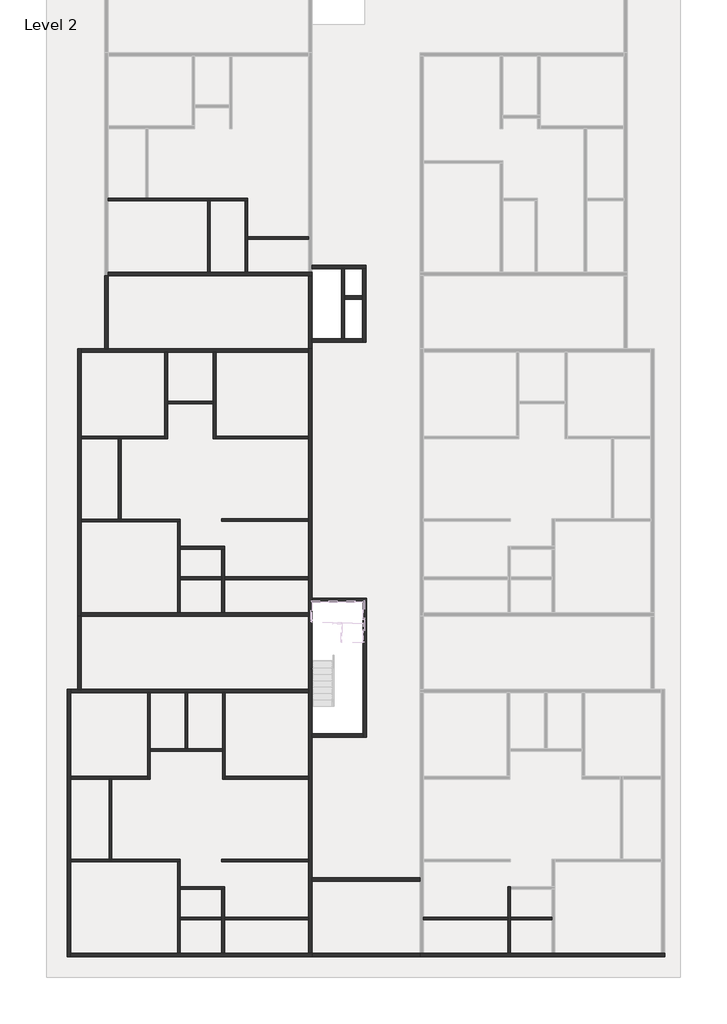
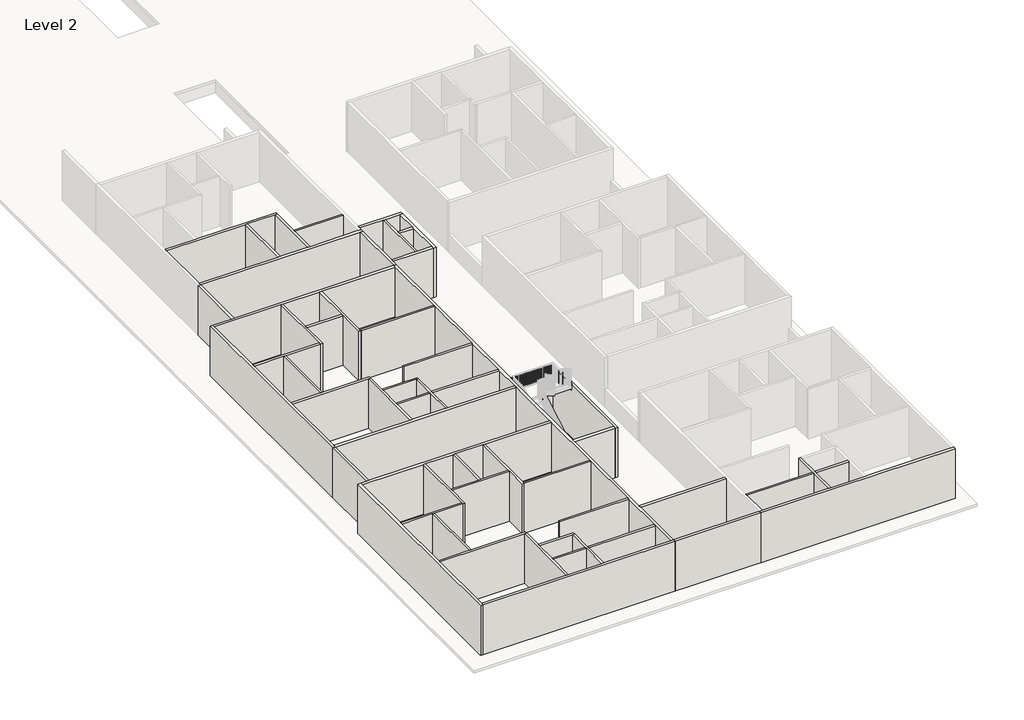
# One storey, part 1 of 8: 55 walls.
"""IFC4 building model written with IfcOpenShell, lengths in millimetres."""

from ifc_helpers import new_model, si_unit, frame, origin, place, context, project, spatial, polyline, outline, extrude, faceted_brep, element, save

model = new_model("IFC4")

# Units and contexts
model_context = context("Model", 3, world=origin())
ifc_project = project(units=[si_unit("LENGTHUNIT", "METRE", prefix="MILLI")], contexts=[model_context])

# Site, building, storey
site = spatial("IfcSite", under=ifc_project)
building = spatial("IfcBuilding", under=site)
storey = spatial("IfcBuildingStorey", under=building, Name="Level 2", Elevation=28282.6172466)

# Walls
placement = place(None, origin())
element("IfcWall", 1, ObjectType="4.5\"", at=placement, inside=storey, context=model_context, shape_type="Brep", body=[
    faceted_brep([(-12531.5544854, -1061.7344126, 28282.6172466), (-8188.1544854, -1061.7344126, 28282.6172466), (-8073.8544854, -1061.7344126, 28282.6172466), (-6549.8544854, -1061.7344126, 28282.6172466), (-6435.5544854, -1061.7344126, 28282.6172466), (-6435.5544854, -1061.7344126, 31330.6172466), (-6549.8544854, -1061.7344126, 31330.6172466), (-8073.8544854, -1061.7344126, 31330.6172466), (-8188.1544854, -1061.7344126, 31330.6172466), (-12531.5544854, -1061.7344126, 31330.6172466), (-12531.5544854, -947.4344126, 28282.6172466), (-12531.5544854, -947.4344126, 31330.6172466), (-10907.2415084, -947.4344126, 31330.6172466), (-10792.9415084, -947.4344126, 31330.6172466), (-6435.5544854, -947.4344126, 31330.6172466), (-6435.5544854, -947.4344126, 28282.6172466), (-10792.9415084, -947.4344126, 28282.6172466), (-10907.2415084, -947.4344126, 28282.6172466)], [[[0, 1, 2, 3, 4, 5, 6, 7, 8, 9]], [[10, 11, 12, 13, 14, 15, 16, 17]], [[4, 3, 2, 1, 0, 10, 17, 16, 15]], [[0, 9, 11, 10]], [[5, 4, 15, 14]], [[9, 8, 7, 6, 5, 14, 13, 12, 11]]]),
])
element("IfcWall", 2, ObjectType="4.5\"", at=placement, inside=storey, context=model_context, shape_type="Brep", body=[
    faceted_brep([(-6549.8544854, -1061.7344126, 28282.6172466), (-6549.8544854, -4185.9344126, 28282.6172466), (-6549.8544854, -4185.9344126, 31330.6172466), (-6549.8544854, -1061.7344126, 31330.6172466), (-6435.5544854, -1061.7344126, 28282.6172466), (-6435.5544854, -1061.7344126, 31330.6172466), (-6435.5544854, -2623.8344126, 31330.6172466), (-6435.5544854, -2738.1344126, 31330.6172466), (-6435.5544854, -4185.9344126, 31330.6172466), (-6435.5544854, -4185.9344126, 28282.6172466), (-6435.5544854, -2738.1344126, 28282.6172466), (-6435.5544854, -2623.8344126, 28282.6172466)], [[[0, 1, 2, 3]], [[4, 5, 6, 7, 8, 9, 10, 11]], [[1, 0, 4, 11, 10, 9]], [[0, 3, 5, 4]], [[2, 1, 9, 8]], [[3, 2, 8, 7, 6, 5]]]),
])
element("IfcWall", 3, ObjectType="4.5\"", at=placement, inside=storey, context=model_context, shape_type="SweptSolid", body=[
    extrude(outline(polyline([(-8188.1544854, -4185.9344126), (-8188.1544854, -1061.7344126), (-8073.8544854, -1061.7344126), (-8073.8544854, -4185.9344126), (-8188.1544854, -4185.9344126)])), frame((0.0, 0.0, 28282.6172466), z_axis=(0.0, 0.0, 1.0), x_axis=(1.0, 0.0, 0.0)), (0.0, 0.0, 1.0), 3048.0),
])
element("IfcWall", 4, ObjectType="4.5\"", at=placement, inside=storey, context=model_context, shape_type="SweptSolid", body=[
    extrude(outline(polyline([(-6435.5544854, -2623.8344126), (-3769.8415084, -2623.8344126), (-3769.8415084, -2738.1344126), (-6435.5544854, -2738.1344126), (-6435.5544854, -2623.8344126)])), frame((0.0, 0.0, 28282.6172466), z_axis=(0.0, 0.0, 1.0), x_axis=(1.0, 0.0, 0.0)), (0.0, 0.0, 1.0), 3048.0),
])
element("IfcWall", 5, ObjectType="4.5\"", at=placement, inside=storey, context=model_context, shape_type="Brep", body=[
    faceted_brep([(-10061.4044854, -7691.1344126, 28282.6172466), (-10061.4044854, -11348.7344126, 28282.6172466), (-10061.4044854, -11463.0344126, 28282.6172466), (-10061.4044854, -11463.0344126, 31330.6172466), (-10061.4044854, -11348.7344126, 31330.6172466), (-10061.4044854, -7691.1344126, 31330.6172466), (-9947.1044854, -7691.1344126, 28282.6172466), (-9947.1044854, -7691.1344126, 31330.6172466), (-9947.1044854, -9824.7344126, 31330.6172466), (-9947.1044854, -9939.0344126, 31330.6172466), (-9947.1044854, -11463.0344126, 31330.6172466), (-9947.1044854, -11463.0344126, 28282.6172466), (-9947.1044854, -9939.0344126, 28282.6172466), (-9947.1044854, -9824.7344126, 28282.6172466)], [[[0, 1, 2, 3, 4, 5]], [[6, 7, 8, 9, 10, 11, 12, 13]], [[2, 1, 0, 6, 13, 12, 11]], [[0, 5, 7, 6]], [[3, 2, 11, 10]], [[5, 4, 3, 10, 9, 8, 7]]]),
])
element("IfcWall", 6, ObjectType="4.5\"", at=placement, inside=storey, context=model_context, shape_type="Brep", body=[
    faceted_brep([(-10061.4044854, -11348.7344126, 28282.6172466), (-13719.0044854, -11348.7344126, 28282.6172466), (-13719.0044854, -11348.7344126, 31330.6172466), (-10061.4044854, -11348.7344126, 31330.6172466), (-10061.4044854, -11463.0344126, 28282.6172466), (-10061.4044854, -11463.0344126, 31330.6172466), (-11980.3915084, -11463.0344126, 31330.6172466), (-12094.6915084, -11463.0344126, 31330.6172466), (-13719.0044854, -11463.0344126, 31330.6172466), (-13719.0044854, -11463.0344126, 28282.6172466), (-12094.6915084, -11463.0344126, 28282.6172466), (-11980.3915084, -11463.0344126, 28282.6172466)], [[[0, 1, 2, 3]], [[4, 5, 6, 7, 8, 9, 10, 11]], [[1, 0, 4, 11, 10, 9]], [[0, 3, 5, 4]], [[2, 1, 9, 8]], [[3, 2, 8, 7, 6, 5]]]),
])
element("IfcWall", 7, ObjectType="4.5\"", at=placement, inside=storey, context=model_context, shape_type="SweptSolid", body=[
    extrude(outline(polyline([(-12094.6915084, -14968.2344126), (-12094.6915084, -11463.0344126), (-11980.3915084, -11463.0344126), (-11980.3915084, -14968.2344126), (-12094.6915084, -14968.2344126)])), frame((0.0, 0.0, 28282.6172466), z_axis=(0.0, 0.0, 1.0), x_axis=(1.0, 0.0, 0.0)), (0.0, 0.0, 1.0), 3048.0),
])
element("IfcWall", 8, ObjectType="4.5\"", at=placement, inside=storey, context=model_context, shape_type="Brep", body=[
    faceted_brep([(-13719.0044854, -15095.2344126, 28282.6172466), (-9510.2415084, -15095.2344126, 28282.6172466), (-9395.9415084, -15095.2344126, 28282.6172466), (-9395.9415084, -15095.2344126, 31330.6172466), (-9510.2415084, -15095.2344126, 31330.6172466), (-13719.0044854, -15095.2344126, 31330.6172466), (-13719.0044854, -14980.9344126, 28282.6172466), (-13719.0044854, -14980.9344126, 31330.6172466), (-9395.9415084, -14980.9344126, 31330.6172466), (-9395.9415084, -14980.9344126, 28282.6172466)], [[[0, 1, 2, 3, 4, 5]], [[6, 7, 8, 9]], [[2, 1, 0, 6, 9]], [[0, 5, 7, 6]], [[3, 2, 9, 8]], [[5, 4, 3, 8, 7]]]),
])
element("IfcWall", 9, ObjectType="4.5\"", at=placement, inside=storey, context=model_context, shape_type="Brep", body=[
    faceted_brep([(-9510.2415084, -15095.2344126, 28282.6172466), (-9510.2415084, -19070.3344126, 28282.6172466), (-9510.2415084, -19070.3344126, 31330.6172466), (-9510.2415084, -15095.2344126, 31330.6172466), (-9395.9415084, -15095.2344126, 28282.6172466), (-9395.9415084, -15095.2344126, 31330.6172466), (-9395.9415084, -16174.7344126, 31330.6172466), (-9395.9415084, -16289.0344126, 31330.6172466), (-9395.9415084, -17508.2344126, 31330.6172466), (-9395.9415084, -17622.5344126, 31330.6172466), (-9395.9415084, -19070.3344126, 31330.6172466), (-9395.9415084, -19070.3344126, 28282.6172466), (-9395.9415084, -17622.5344126, 28282.6172466), (-9395.9415084, -17508.2344126, 28282.6172466), (-9395.9415084, -16289.0344126, 28282.6172466), (-9395.9415084, -16174.7344126, 28282.6172466)], [[[0, 1, 2, 3]], [[4, 5, 6, 7, 8, 9, 10, 11, 12, 13, 14, 15]], [[1, 0, 4, 15, 14, 13, 12, 11]], [[0, 3, 5, 4]], [[2, 1, 11, 10]], [[3, 2, 10, 9, 8, 7, 6, 5]]]),
])
element("IfcWall", 10, ObjectType="4.5\"", at=placement, inside=storey, context=model_context, shape_type="Brep", body=[
    faceted_brep([(-9395.9415084, -16289.0344126, 28282.6172466), (-7567.1415084, -16289.0344126, 28282.6172466), (-7452.8415084, -16289.0344126, 28282.6172466), (-7452.8415084, -16289.0344126, 31330.6172466), (-7567.1415084, -16289.0344126, 31330.6172466), (-9395.9415084, -16289.0344126, 31330.6172466), (-9395.9415084, -16174.7344126, 28282.6172466), (-9395.9415084, -16174.7344126, 31330.6172466), (-7452.8415084, -16174.7344126, 31330.6172466), (-7452.8415084, -16174.7344126, 28282.6172466)], [[[0, 1, 2, 3, 4, 5]], [[6, 7, 8, 9]], [[2, 1, 0, 6, 9]], [[0, 5, 7, 6]], [[3, 2, 9, 8]], [[5, 4, 3, 8, 7]]]),
])
element("IfcWall", 11, ObjectType="4.5\"", at=placement, inside=storey, context=model_context, shape_type="Brep", body=[
    faceted_brep([(-7567.1415084, -16289.0344126, 28282.6172466), (-7567.1415084, -17508.2344126, 28282.6172466), (-7567.1415084, -17622.5344126, 28282.6172466), (-7567.1415084, -19070.3344126, 28282.6172466), (-7567.1415084, -19070.3344126, 31330.6172466), (-7567.1415084, -17622.5344126, 31330.6172466), (-7567.1415084, -17508.2344126, 31330.6172466), (-7567.1415084, -16289.0344126, 31330.6172466), (-7452.8415084, -16289.0344126, 28282.6172466), (-7452.8415084, -16289.0344126, 31330.6172466), (-7452.8415084, -17508.2344126, 31330.6172466), (-7452.8415084, -17622.5344126, 31330.6172466), (-7452.8415084, -19070.3344126, 31330.6172466), (-7452.8415084, -19070.3344126, 28282.6172466), (-7452.8415084, -17622.5344126, 28282.6172466), (-7452.8415084, -17508.2344126, 28282.6172466)], [[[0, 1, 2, 3, 4, 5, 6, 7]], [[8, 9, 10, 11, 12, 13, 14, 15]], [[3, 2, 1, 0, 8, 15, 14, 13]], [[0, 7, 9, 8]], [[4, 3, 13, 12]], [[7, 6, 5, 4, 12, 11, 10, 9]]]),
])
element("IfcWall", 12, ObjectType="4.5\"", at=placement, inside=storey, context=model_context, shape_type="SweptSolid", body=[
    extrude(outline(polyline([(-7567.1415084, -17622.5344126), (-9395.9415084, -17622.5344126), (-9395.9415084, -17508.2344126), (-7567.1415084, -17508.2344126), (-7567.1415084, -17622.5344126)])), frame((0.0, 0.0, 28282.6172466), z_axis=(0.0, 0.0, 1.0), x_axis=(1.0, 0.0, 0.0)), (0.0, 0.0, 1.0), 3048.0),
])
element("IfcWall", 13, ObjectType="4.5\"", at=placement, inside=storey, context=model_context, shape_type="SweptSolid", body=[
    extrude(outline(polyline([(-3769.8415084, -17622.5344126), (-7452.8415084, -17622.5344126), (-7452.8415084, -17508.2344126), (-3769.8415084, -17508.2344126), (-3769.8415084, -17622.5344126)])), frame((0.0, 0.0, 28282.6172466), z_axis=(0.0, 0.0, 1.0), x_axis=(1.0, 0.0, 0.0)), (0.0, 0.0, 1.0), 3048.0),
])
element("IfcWall", 14, ObjectType="4.5\"", at=placement, inside=storey, context=model_context, shape_type="SweptSolid", body=[
    extrude(outline(polyline([(-7567.1415084, -14968.2344126), (-3769.8415084, -14968.2344126), (-3769.8415084, -15082.5344126), (-7567.1415084, -15082.5344126), (-7567.1415084, -14968.2344126)])), frame((0.0, 0.0, 28282.6172466), z_axis=(0.0, 0.0, 1.0), x_axis=(1.0, 0.0, 0.0)), (0.0, 0.0, 1.0), 3048.0),
])
element("IfcWall", 15, ObjectType="4.5\"", at=placement, inside=storey, context=model_context, shape_type="SweptSolid", body=[
    extrude(outline(polyline([(-7940.5044854, -9939.0344126), (-9947.1044854, -9939.0344126), (-9947.1044854, -9824.7344126), (-7940.5044854, -9824.7344126), (-7940.5044854, -9939.0344126)])), frame((0.0, 0.0, 28282.6172466), z_axis=(0.0, 0.0, 1.0), x_axis=(1.0, 0.0, 0.0)), (0.0, 0.0, 1.0), 3048.0),
])
element("IfcWall", 16, ObjectType="4.5\"", at=placement, inside=storey, context=model_context, shape_type="Brep", body=[
    faceted_brep([(-7940.5044854, -7691.1344126, 28282.6172466), (-7940.5044854, -9824.7344126, 28282.6172466), (-7940.5044854, -9939.0344126, 28282.6172466), (-7940.5044854, -11463.0344126, 28282.6172466), (-7940.5044854, -11463.0344126, 31330.6172466), (-7940.5044854, -9939.0344126, 31330.6172466), (-7940.5044854, -9824.7344126, 31330.6172466), (-7940.5044854, -7691.1344126, 31330.6172466), (-7826.2044854, -7691.1344126, 28282.6172466), (-7826.2044854, -7691.1344126, 31330.6172466), (-7826.2044854, -11348.7344126, 31330.6172466), (-7826.2044854, -11463.0344126, 31330.6172466), (-7826.2044854, -11463.0344126, 28282.6172466), (-7826.2044854, -11348.7344126, 28282.6172466)], [[[0, 1, 2, 3, 4, 5, 6, 7]], [[8, 9, 10, 11, 12, 13]], [[3, 2, 1, 0, 8, 13, 12]], [[0, 7, 9, 8]], [[4, 3, 12, 11]], [[7, 6, 5, 4, 11, 10, 9]]]),
])
element("IfcWall", 17, ObjectType="4.5\"", at=placement, inside=storey, context=model_context, shape_type="SweptSolid", body=[
    extrude(outline(polyline([(-3769.8415084, -11463.0344126), (-7826.2044854, -11463.0344126), (-7826.2044854, -11348.7344126), (-3769.8415084, -11348.7344126), (-3769.8415084, -11463.0344126)])), frame((0.0, 0.0, 28282.6172466), z_axis=(0.0, 0.0, 1.0), x_axis=(1.0, 0.0, 0.0)), (0.0, 0.0, 1.0), 3048.0),
])
element("IfcWall", 18, ObjectType="4.5\"", at=placement, inside=storey, context=model_context, shape_type="Brep", body=[
    faceted_brep([(-10818.3415084, -22575.5344126, 28282.6172466), (-10818.3415084, -26233.1344126, 28282.6172466), (-10818.3415084, -26347.4344126, 28282.6172466), (-10818.3415084, -26347.4344126, 31330.6172466), (-10818.3415084, -26233.1344126, 31330.6172466), (-10818.3415084, -22575.5344126, 31330.6172466), (-10704.0415084, -22575.5344126, 28282.6172466), (-10704.0415084, -22575.5344126, 31330.6172466), (-10704.0415084, -25013.9344126, 31330.6172466), (-10704.0415084, -25128.2344126, 31330.6172466), (-10704.0415084, -26347.4344126, 31330.6172466), (-10704.0415084, -26347.4344126, 28282.6172466), (-10704.0415084, -25128.2344126, 28282.6172466), (-10704.0415084, -25013.9344126, 28282.6172466)], [[[0, 1, 2, 3, 4, 5]], [[6, 7, 8, 9, 10, 11, 12, 13]], [[2, 1, 0, 6, 13, 12, 11]], [[0, 5, 7, 6]], [[3, 2, 11, 10]], [[5, 4, 3, 10, 9, 8, 7]]]),
])
element("IfcWall", 19, ObjectType="4.5\"", at=placement, inside=storey, context=model_context, shape_type="Brep", body=[
    faceted_brep([(-10818.3415084, -26233.1344126, 28282.6172466), (-14171.1415084, -26233.1344126, 28282.6172466), (-14171.1415084, -26233.1344126, 31330.6172466), (-10818.3415084, -26233.1344126, 31330.6172466), (-10818.3415084, -26347.4344126, 28282.6172466), (-10818.3415084, -26347.4344126, 31330.6172466), (-12380.4415084, -26347.4344126, 31330.6172466), (-12494.7415084, -26347.4344126, 31330.6172466), (-14171.1415084, -26347.4344126, 31330.6172466), (-14171.1415084, -26347.4344126, 28282.6172466), (-12494.7415084, -26347.4344126, 28282.6172466), (-12380.4415084, -26347.4344126, 28282.6172466)], [[[0, 1, 2, 3]], [[4, 5, 6, 7, 8, 9, 10, 11]], [[1, 0, 4, 11, 10, 9]], [[0, 3, 5, 4]], [[2, 1, 9, 8]], [[3, 2, 8, 7, 6, 5]]]),
])
element("IfcWall", 20, ObjectType="4.5\"", at=placement, inside=storey, context=model_context, shape_type="SweptSolid", body=[
    extrude(outline(polyline([(-9180.0415084, -25013.9344126), (-9180.0415084, -22575.5344126), (-9065.7415084, -22575.5344126), (-9065.7415084, -25013.9344126), (-9180.0415084, -25013.9344126)])), frame((0.0, 0.0, 28282.6172466), z_axis=(0.0, 0.0, 1.0), x_axis=(1.0, 0.0, 0.0)), (0.0, 0.0, 1.0), 3048.0),
])
element("IfcWall", 21, ObjectType="4.5\"", at=placement, inside=storey, context=model_context, shape_type="Brep", body=[
    faceted_brep([(-10704.0415084, -25128.2344126, 28282.6172466), (-7541.7415084, -25128.2344126, 28282.6172466), (-7541.7415084, -25128.2344126, 31330.6172466), (-10704.0415084, -25128.2344126, 31330.6172466), (-10704.0415084, -25013.9344126, 28282.6172466), (-10704.0415084, -25013.9344126, 31330.6172466), (-9180.0415084, -25013.9344126, 31330.6172466), (-9065.7415084, -25013.9344126, 31330.6172466), (-7541.7415084, -25013.9344126, 31330.6172466), (-7541.7415084, -25013.9344126, 28282.6172466), (-9065.7415084, -25013.9344126, 28282.6172466), (-9180.0415084, -25013.9344126, 28282.6172466)], [[[0, 1, 2, 3]], [[4, 5, 6, 7, 8, 9, 10, 11]], [[1, 0, 4, 11, 10, 9]], [[0, 3, 5, 4]], [[2, 1, 9, 8]], [[3, 2, 8, 7, 6, 5]]]),
])
element("IfcWall", 22, ObjectType="4.5\"", at=placement, inside=storey, context=model_context, shape_type="Brep", body=[
    faceted_brep([(-7541.7415084, -22575.5344126, 28282.6172466), (-7541.7415084, -25013.9344126, 28282.6172466), (-7541.7415084, -25128.2344126, 28282.6172466), (-7541.7415084, -26347.4344126, 28282.6172466), (-7541.7415084, -26347.4344126, 31330.6172466), (-7541.7415084, -25128.2344126, 31330.6172466), (-7541.7415084, -25013.9344126, 31330.6172466), (-7541.7415084, -22575.5344126, 31330.6172466), (-7427.4415084, -22575.5344126, 28282.6172466), (-7427.4415084, -22575.5344126, 31330.6172466), (-7427.4415084, -26233.1344126, 31330.6172466), (-7427.4415084, -26347.4344126, 31330.6172466), (-7427.4415084, -26347.4344126, 28282.6172466), (-7427.4415084, -26233.1344126, 28282.6172466)], [[[0, 1, 2, 3, 4, 5, 6, 7]], [[8, 9, 10, 11, 12, 13]], [[3, 2, 1, 0, 8, 13, 12]], [[0, 7, 9, 8]], [[4, 3, 12, 11]], [[7, 6, 5, 4, 11, 10, 9]]]),
])
element("IfcWall", 23, ObjectType="4.5\"", at=placement, inside=storey, context=model_context, shape_type="SweptSolid", body=[
    extrude(outline(polyline([(-3769.8415084, -26347.4344126), (-7427.4415084, -26347.4344126), (-7427.4415084, -26233.1344126), (-3769.8415084, -26233.1344126), (-3769.8415084, -26347.4344126)])), frame((0.0, 0.0, 28282.6172466), z_axis=(0.0, 0.0, 1.0), x_axis=(1.0, 0.0, 0.0)), (0.0, 0.0, 1.0), 3048.0),
])
element("IfcWall", 24, ObjectType="4.5\"", at=placement, inside=storey, context=model_context, shape_type="SweptSolid", body=[
    extrude(outline(polyline([(-12494.7415084, -29852.6344126), (-12494.7415084, -26347.4344126), (-12380.4415084, -26347.4344126), (-12380.4415084, -29852.6344126), (-12494.7415084, -29852.6344126)])), frame((0.0, 0.0, 28282.6172466), z_axis=(0.0, 0.0, 1.0), x_axis=(1.0, 0.0, 0.0)), (0.0, 0.0, 1.0), 3048.0),
])
element("IfcWall", 25, ObjectType="4.5\"", at=placement, inside=storey, context=model_context, shape_type="Brep", body=[
    faceted_brep([(-14171.1415084, -29966.9344126, 28282.6172466), (-9510.2415084, -29966.9344126, 28282.6172466), (-9395.9415084, -29966.9344126, 28282.6172466), (-9395.9415084, -29966.9344126, 31330.6172466), (-9510.2415084, -29966.9344126, 31330.6172466), (-14171.1415084, -29966.9344126, 31330.6172466), (-14171.1415084, -29852.6344126, 28282.6172466), (-14171.1415084, -29852.6344126, 31330.6172466), (-12494.7415084, -29852.6344126, 31330.6172466), (-12380.4415084, -29852.6344126, 31330.6172466), (-9395.9415084, -29852.6344126, 31330.6172466), (-9395.9415084, -29852.6344126, 28282.6172466), (-12380.4415084, -29852.6344126, 28282.6172466), (-12494.7415084, -29852.6344126, 28282.6172466)], [[[0, 1, 2, 3, 4, 5]], [[6, 7, 8, 9, 10, 11, 12, 13]], [[2, 1, 0, 6, 13, 12, 11]], [[0, 5, 7, 6]], [[3, 2, 11, 10]], [[5, 4, 3, 10, 9, 8, 7]]]),
])
element("IfcWall", 26, ObjectType="4.5\"", at=placement, inside=storey, context=model_context, shape_type="Brep", body=[
    faceted_brep([(-9510.2415084, -29966.9344126, 28282.6172466), (-9510.2415084, -33954.7344126, 28282.6172466), (-9510.2415084, -33954.7344126, 31330.6172466), (-9510.2415084, -29966.9344126, 31330.6172466), (-9395.9415084, -29966.9344126, 28282.6172466), (-9395.9415084, -29966.9344126, 31330.6172466), (-9395.9415084, -31059.1344126, 31330.6172466), (-9395.9415084, -31173.4344126, 31330.6172466), (-9395.9415084, -32392.6344126, 31330.6172466), (-9395.9415084, -32506.9344126, 31330.6172466), (-9395.9415084, -33954.7344126, 31330.6172466), (-9395.9415084, -33954.7344126, 28282.6172466), (-9395.9415084, -32506.9344126, 28282.6172466), (-9395.9415084, -32392.6344126, 28282.6172466), (-9395.9415084, -31173.4344126, 28282.6172466), (-9395.9415084, -31059.1344126, 28282.6172466)], [[[0, 1, 2, 3]], [[4, 5, 6, 7, 8, 9, 10, 11, 12, 13, 14, 15]], [[1, 0, 4, 15, 14, 13, 12, 11]], [[0, 3, 5, 4]], [[2, 1, 11, 10]], [[3, 2, 10, 9, 8, 7, 6, 5]]]),
])
element("IfcWall", 27, ObjectType="4.5\"", at=placement, inside=storey, context=model_context, shape_type="Brep", body=[
    faceted_brep([(-9395.9415084, -31173.4344126, 28282.6172466), (-7567.1415084, -31173.4344126, 28282.6172466), (-7452.8415084, -31173.4344126, 28282.6172466), (-7452.8415084, -31173.4344126, 31330.6172466), (-7567.1415084, -31173.4344126, 31330.6172466), (-9395.9415084, -31173.4344126, 31330.6172466), (-9395.9415084, -31059.1344126, 28282.6172466), (-9395.9415084, -31059.1344126, 31330.6172466), (-7452.8415084, -31059.1344126, 31330.6172466), (-7452.8415084, -31059.1344126, 28282.6172466)], [[[0, 1, 2, 3, 4, 5]], [[6, 7, 8, 9]], [[2, 1, 0, 6, 9]], [[0, 5, 7, 6]], [[3, 2, 9, 8]], [[5, 4, 3, 8, 7]]]),
])
element("IfcWall", 28, ObjectType="4.5\"", at=placement, inside=storey, context=model_context, shape_type="Brep", body=[
    faceted_brep([(-7567.1415084, -31173.4344126, 28282.6172466), (-7567.1415084, -32392.6344126, 28282.6172466), (-7567.1415084, -32506.9344126, 28282.6172466), (-7567.1415084, -33954.7344126, 28282.6172466), (-7567.1415084, -33954.7344126, 31330.6172466), (-7567.1415084, -32506.9344126, 31330.6172466), (-7567.1415084, -32392.6344126, 31330.6172466), (-7567.1415084, -31173.4344126, 31330.6172466), (-7452.8415084, -31173.4344126, 28282.6172466), (-7452.8415084, -31173.4344126, 31330.6172466), (-7452.8415084, -32392.6344126, 31330.6172466), (-7452.8415084, -32506.9344126, 31330.6172466), (-7452.8415084, -33954.7344126, 31330.6172466), (-7452.8415084, -33954.7344126, 28282.6172466), (-7452.8415084, -32506.9344126, 28282.6172466), (-7452.8415084, -32392.6344126, 28282.6172466)], [[[0, 1, 2, 3, 4, 5, 6, 7]], [[8, 9, 10, 11, 12, 13, 14, 15]], [[3, 2, 1, 0, 8, 15, 14, 13]], [[0, 7, 9, 8]], [[4, 3, 13, 12]], [[7, 6, 5, 4, 12, 11, 10, 9]]]),
])
element("IfcWall", 29, ObjectType="4.5\"", at=placement, inside=storey, context=model_context, shape_type="SweptSolid", body=[
    extrude(outline(polyline([(-3769.8415084, -32392.6344126), (-3769.8415084, -32506.9344126), (-7452.8415084, -32506.9344126), (-7452.8415084, -32392.6344126), (-3769.8415084, -32392.6344126)])), frame((0.0, 0.0, 28282.6172466), z_axis=(0.0, 0.0, 1.0), x_axis=(1.0, 0.0, 0.0)), (0.0, 0.0, 1.0), 3048.0),
    extrude(outline(polyline([(-9395.9415084, -32506.9344126), (-9395.9415084, -32392.6344126), (-7567.1415084, -32392.6344126), (-7567.1415084, -32506.9344126), (-9395.9415084, -32506.9344126)])), frame((0.0, 0.0, 28282.6172466), z_axis=(0.0, 0.0, 1.0), x_axis=(1.0, 0.0, 0.0)), (0.0, 0.0, 1.0), 3048.0),
])
element("IfcWall", 30, ObjectType="4.5\"", at=placement, inside=storey, context=model_context, shape_type="SweptSolid", body=[
    extrude(outline(polyline([(-7567.1415084, -29852.6344126), (-3769.8415084, -29852.6344126), (-3769.8415084, -29966.9344126), (-7567.1415084, -29966.9344126), (-7567.1415084, -29852.6344126)])), frame((0.0, 0.0, 28282.6172466), z_axis=(0.0, 0.0, 1.0), x_axis=(1.0, 0.0, 0.0)), (0.0, 0.0, 1.0), 3048.0),
])
element("IfcWall", 31, ObjectType="4.5\"", at=placement, inside=storey, context=model_context, shape_type="SweptSolid", body=[
    extrude(outline(polyline([(4942.3584916, -32506.9344126), (1259.3584916, -32506.9344126), (1259.3584916, -32392.6344126), (4942.3584916, -32392.6344126), (4942.3584916, -32506.9344126)])), frame((0.0, 0.0, 28282.6172466), z_axis=(0.0, 0.0, 1.0), x_axis=(1.0, 0.0, 0.0)), (0.0, 0.0, 1.0), 3048.0),
])
element("IfcWall", 32, ObjectType="4.5\"", at=placement, inside=storey, context=model_context, shape_type="Brep", body=[
    faceted_brep([(4942.3584916, -31059.1344126, 28282.6172466), (4942.3584916, -32392.6344126, 28282.6172466), (4942.3584916, -32506.9344126, 28282.6172466), (4942.3584916, -33954.7344126, 28282.6172466), (4942.3584916, -33954.7344126, 31330.6172466), (4942.3584916, -32506.9344126, 31330.6172466), (4942.3584916, -32392.6344126, 31330.6172466), (4942.3584916, -31059.1344126, 31330.6172466), (5056.6584916, -31059.1344126, 28282.6172466), (5056.6584916, -31059.1344126, 31330.6172466), (5056.6584916, -31173.4344126, 31330.6172466), (5056.6584916, -32392.6344126, 31330.6172466), (5056.6584916, -32506.9344126, 31330.6172466), (5056.6584916, -33954.7344126, 31330.6172466), (5056.6584916, -33954.7344126, 28282.6172466), (5056.6584916, -32506.9344126, 28282.6172466), (5056.6584916, -32392.6344126, 28282.6172466), (5056.6584916, -31173.4344126, 28282.6172466)], [[[0, 1, 2, 3, 4, 5, 6, 7]], [[8, 9, 10, 11, 12, 13, 14, 15, 16, 17]], [[3, 2, 1, 0, 8, 17, 16, 15, 14]], [[4, 3, 14, 13]], [[0, 7, 9, 8]], [[7, 6, 5, 4, 13, 12, 11, 10, 9]]]),
])
element("IfcWall", 33, ObjectType="4.5\"", at=placement, inside=storey, context=model_context, shape_type="SweptSolid", body=[
    extrude(outline(polyline([(6885.4584916, -32506.9344126), (5056.6584916, -32506.9344126), (5056.6584916, -32392.6344126), (6885.4584916, -32392.6344126), (6885.4584916, -32506.9344126)])), frame((0.0, 0.0, 28282.6172466), z_axis=(0.0, 0.0, 1.0), x_axis=(1.0, 0.0, 0.0)), (0.0, 0.0, 1.0), 3048.0),
])
element("IfcWall", 34, ObjectType="4.5\"", at=placement, inside=storey, context=model_context, shape_type="Brep", body=[
    faceted_brep([(-2207.6738684, -7082.6751812, 28282.6172466), (-2207.6738684, -5366.3479894, 28282.6172466), (-2207.6738684, -5213.9479894, 28282.6172466), (-2207.6738684, -4034.6751812, 28282.6172466), (-2207.6738684, -4034.6751812, 31330.6172466), (-2207.6738684, -5213.9479894, 31330.6172466), (-2207.6738684, -5366.3479894, 31330.6172466), (-2207.6738684, -7082.6751812, 31330.6172466), (-2321.9738684, -7082.6751812, 28282.6172466), (-2321.9738684, -7082.6751812, 31330.6172466), (-2321.9738684, -4034.6751812, 31330.6172466), (-2321.9738684, -4034.6751812, 28282.6172466)], [[[0, 1, 2, 3, 4, 5, 6, 7]], [[8, 9, 10, 11]], [[3, 2, 1, 0, 8, 11]], [[7, 6, 5, 4, 10, 9]], [[4, 3, 11, 10]], [[0, 7, 9, 8]]]),
])
element("IfcWall", 35, ObjectType="6\"", at=placement, inside=storey, context=model_context, shape_type="Brep", body=[
    faceted_brep([(-12531.5544854, -4338.3344126, 28282.6172466), (-3769.8415084, -4338.3344126, 28282.6172466), (-3617.4415084, -4338.3344126, 28282.6172466), (-3617.4415084, -4338.3344126, 31330.6172466), (-3769.8415084, -4338.3344126, 31330.6172466), (-12531.5544854, -4338.3344126, 31330.6172466), (-12531.5544854, -4185.9344126, 28282.6172466), (-12531.5544854, -4185.9344126, 31330.6172466), (-8188.1544854, -4185.9344126, 31330.6172466), (-8073.8544854, -4185.9344126, 31330.6172466), (-6549.8544854, -4185.9344126, 31330.6172466), (-6435.5544854, -4185.9344126, 31330.6172466), (-3769.8415084, -4185.9344126, 31330.6172466), (-3617.4415084, -4185.9344126, 31330.6172466), (-3617.4415084, -4185.9344126, 28282.6172466), (-3769.8415084, -4185.9344126, 28282.6172466), (-6435.5544854, -4185.9344126, 28282.6172466), (-6549.8544854, -4185.9344126, 28282.6172466), (-8073.8544854, -4185.9344126, 28282.6172466), (-8188.1544854, -4185.9344126, 28282.6172466)], [[[0, 1, 2, 3, 4, 5]], [[6, 7, 8, 9, 10, 11, 12, 13, 14, 15, 16, 17, 18, 19]], [[2, 1, 0, 6, 19, 18, 17, 16, 15, 14]], [[0, 5, 7, 6]], [[3, 2, 14, 13]], [[5, 4, 3, 13, 12, 11, 10, 9, 8, 7]]]),
])
element("IfcWall", 36, ObjectType="6\"", at=placement, inside=storey, context=model_context, shape_type="Brep", body=[
    faceted_brep([(-13871.4044854, -7538.7344126, 28282.6172466), (-13871.4044854, -19222.7344126, 28282.6172466), (-13871.4044854, -19222.7344126, 31330.6172466), (-13871.4044854, -7538.7344126, 31330.6172466), (-13719.0044854, -7538.7344126, 28282.6172466), (-13719.0044854, -7538.7344126, 31330.6172466), (-13719.0044854, -7691.1344126, 31330.6172466), (-13719.0044854, -11348.7344126, 31330.6172466), (-13719.0044854, -11463.0344126, 31330.6172466), (-13719.0044854, -14980.9344126, 31330.6172466), (-13719.0044854, -15095.2344126, 31330.6172466), (-13719.0044854, -19070.3344126, 31330.6172466), (-13719.0044854, -19222.7344126, 31330.6172466), (-13719.0044854, -19222.7344126, 28282.6172466), (-13719.0044854, -19070.3344126, 28282.6172466), (-13719.0044854, -15095.2344126, 28282.6172466), (-13719.0044854, -14980.9344126, 28282.6172466), (-13719.0044854, -11463.0344126, 28282.6172466), (-13719.0044854, -11348.7344126, 28282.6172466), (-13719.0044854, -7691.1344126, 28282.6172466)], [[[0, 1, 2, 3]], [[4, 5, 6, 7, 8, 9, 10, 11, 12, 13, 14, 15, 16, 17, 18, 19]], [[1, 0, 4, 19, 18, 17, 16, 15, 14, 13]], [[2, 1, 13, 12]], [[0, 3, 5, 4]], [[3, 2, 12, 11, 10, 9, 8, 7, 6, 5]]]),
])
element("IfcWall", 37, ObjectType="6\"", at=placement, inside=storey, context=model_context, shape_type="Brep", body=[
    faceted_brep([(-13719.0044854, -19222.7344126, 28282.6172466), (-3769.8415084, -19222.7344126, 28282.6172466), (-3769.8415084, -19222.7344126, 31330.6172466), (-13719.0044854, -19222.7344126, 31330.6172466), (-13719.0044854, -19070.3344126, 28282.6172466), (-13719.0044854, -19070.3344126, 31330.6172466), (-9510.2415084, -19070.3344126, 31330.6172466), (-9395.9415084, -19070.3344126, 31330.6172466), (-7567.1415084, -19070.3344126, 31330.6172466), (-7452.8415084, -19070.3344126, 31330.6172466), (-3769.8415084, -19070.3344126, 31330.6172466), (-3769.8415084, -19070.3344126, 28282.6172466), (-7452.8415084, -19070.3344126, 28282.6172466), (-7567.1415084, -19070.3344126, 28282.6172466), (-9395.9415084, -19070.3344126, 28282.6172466), (-9510.2415084, -19070.3344126, 28282.6172466)], [[[0, 1, 2, 3]], [[4, 5, 6, 7, 8, 9, 10, 11, 12, 13, 14, 15]], [[1, 0, 4, 15, 14, 13, 12, 11]], [[0, 3, 5, 4]], [[2, 1, 11, 10]], [[3, 2, 10, 9, 8, 7, 6, 5]]]),
])
element("IfcWall", 38, ObjectType="6\"", at=placement, inside=storey, context=model_context, shape_type="Brep", body=[
    faceted_brep([(-3617.4415084, -33954.7344126, 28282.6172466), (-3617.4415084, -30820.9325185, 28282.6172466), (-3617.4415084, -30668.5325185, 28282.6172466), (-3617.4415084, -24525.9851539, 28282.6172466), (-3617.4415084, -24373.5851539, 28282.6172466), (-3617.4415084, -18582.3851539, 28282.6172466), (-3617.4415084, -18429.9851539, 28282.6172466), (-3617.4415084, -7538.7344126, 28282.6172466), (-3617.4415084, -7538.7344126, 31330.6172466), (-3617.4415084, -18429.9851539, 31330.6172466), (-3617.4415084, -18582.3851539, 31330.6172466), (-3617.4415084, -24373.5851539, 31330.6172466), (-3617.4415084, -24525.9851539, 31330.6172466), (-3617.4415084, -30668.5325185, 31330.6172466), (-3617.4415084, -30820.9325185, 31330.6172466), (-3617.4415084, -33954.7344126, 31330.6172466), (-3769.8415084, -33954.7344126, 28282.6172466), (-3769.8415084, -33954.7344126, 31330.6172466), (-3769.8415084, -32506.9344126, 31330.6172466), (-3769.8415084, -32392.6344126, 31330.6172466), (-3769.8415084, -29966.9344126, 31330.6172466), (-3769.8415084, -29852.6344126, 31330.6172466), (-3769.8415084, -26347.4344126, 31330.6172466), (-3769.8415084, -26233.1344126, 31330.6172466), (-3769.8415084, -22575.5344126, 31330.6172466), (-3769.8415084, -22423.1344126, 31330.6172466), (-3769.8415084, -19222.7344126, 31330.6172466), (-3769.8415084, -19070.3344126, 31330.6172466), (-3769.8415084, -17622.5344126, 31330.6172466), (-3769.8415084, -17508.2344126, 31330.6172466), (-3769.8415084, -15082.5344126, 31330.6172466), (-3769.8415084, -14968.2344126, 31330.6172466), (-3769.8415084, -11463.0344126, 31330.6172466), (-3769.8415084, -11348.7344126, 31330.6172466), (-3769.8415084, -7691.1344126, 31330.6172466), (-3769.8415084, -7538.7344126, 31330.6172466), (-3769.8415084, -7538.7344126, 28282.6172466), (-3769.8415084, -7691.1344126, 28282.6172466), (-3769.8415084, -11348.7344126, 28282.6172466), (-3769.8415084, -11463.0344126, 28282.6172466), (-3769.8415084, -14968.2344126, 28282.6172466), (-3769.8415084, -15082.5344126, 28282.6172466), (-3769.8415084, -17508.2344126, 28282.6172466), (-3769.8415084, -17622.5344126, 28282.6172466), (-3769.8415084, -19070.3344126, 28282.6172466), (-3769.8415084, -19222.7344126, 28282.6172466), (-3769.8415084, -22423.1344126, 28282.6172466), (-3769.8415084, -22575.5344126, 28282.6172466), (-3769.8415084, -26233.1344126, 28282.6172466), (-3769.8415084, -26347.4344126, 28282.6172466), (-3769.8415084, -29852.6344126, 28282.6172466), (-3769.8415084, -29966.9344126, 28282.6172466), (-3769.8415084, -32392.6344126, 28282.6172466), (-3769.8415084, -32506.9344126, 28282.6172466)], [[[0, 1, 2, 3, 4, 5, 6, 7, 8, 9, 10, 11, 12, 13, 14, 15]], [[16, 17, 18, 19, 20, 21, 22, 23, 24, 25, 26, 27, 28, 29, 30, 31, 32, 33, 34, 35, 36, 37, 38, 39, 40, 41, 42, 43, 44, 45, 46, 47, 48, 49, 50, 51, 52, 53]], [[7, 6, 5, 4, 3, 2, 1, 0, 16, 53, 52, 51, 50, 49, 48, 47, 46, 45, 44, 43, 42, 41, 40, 39, 38, 37, 36]], [[8, 7, 36, 35]], [[0, 15, 17, 16]], [[15, 14, 13, 12, 11, 10, 9, 8, 35, 34, 33, 32, 31, 30, 29, 28, 27, 26, 25, 24, 23, 22, 21, 20, 19, 18, 17]]]),
])
element("IfcWall", 39, ObjectType="6\"", at=placement, inside=storey, context=model_context, shape_type="Brep", body=[
    faceted_brep([(-3769.8415084, -7538.7344126, 28282.6172466), (-12531.5544854, -7538.7344126, 28282.6172466), (-12683.9544854, -7538.7344126, 28282.6172466), (-13719.0044854, -7538.7344126, 28282.6172466), (-13719.0044854, -7538.7344126, 31330.6172466), (-12683.9544854, -7538.7344126, 31330.6172466), (-12531.5544854, -7538.7344126, 31330.6172466), (-3769.8415084, -7538.7344126, 31330.6172466), (-3769.8415084, -7691.1344126, 28282.6172466), (-3769.8415084, -7691.1344126, 31330.6172466), (-7826.2044854, -7691.1344126, 31330.6172466), (-7940.5044854, -7691.1344126, 31330.6172466), (-9947.1044854, -7691.1344126, 31330.6172466), (-10061.4044854, -7691.1344126, 31330.6172466), (-13719.0044854, -7691.1344126, 31330.6172466), (-13719.0044854, -7691.1344126, 28282.6172466), (-10061.4044854, -7691.1344126, 28282.6172466), (-9947.1044854, -7691.1344126, 28282.6172466), (-7940.5044854, -7691.1344126, 28282.6172466), (-7826.2044854, -7691.1344126, 28282.6172466)], [[[0, 1, 2, 3, 4, 5, 6, 7]], [[8, 9, 10, 11, 12, 13, 14, 15, 16, 17, 18, 19]], [[3, 2, 1, 0, 8, 19, 18, 17, 16, 15]], [[0, 7, 9, 8]], [[4, 3, 15, 14]], [[7, 6, 5, 4, 14, 13, 12, 11, 10, 9]]]),
])
element("IfcWall", 40, ObjectType="6\"", at=placement, inside=storey, context=model_context, shape_type="Brep", body=[
    faceted_brep([(-14323.5415084, -22423.1344126, 28282.6172466), (-14323.5415084, -34107.1344126, 28282.6172466), (-14323.5415084, -34107.1344126, 31330.6172466), (-14323.5415084, -22423.1344126, 31330.6172466), (-14171.1415084, -22423.1344126, 28282.6172466), (-14171.1415084, -22423.1344126, 31330.6172466), (-14171.1415084, -22575.5344126, 31330.6172466), (-14171.1415084, -26233.1344126, 31330.6172466), (-14171.1415084, -26347.4344126, 31330.6172466), (-14171.1415084, -29852.6344126, 31330.6172466), (-14171.1415084, -29966.9344126, 31330.6172466), (-14171.1415084, -33954.7344126, 31330.6172466), (-14171.1415084, -34107.1344126, 31330.6172466), (-14171.1415084, -34107.1344126, 28282.6172466), (-14171.1415084, -33954.7344126, 28282.6172466), (-14171.1415084, -29966.9344126, 28282.6172466), (-14171.1415084, -29852.6344126, 28282.6172466), (-14171.1415084, -26347.4344126, 28282.6172466), (-14171.1415084, -26233.1344126, 28282.6172466), (-14171.1415084, -22575.5344126, 28282.6172466)], [[[0, 1, 2, 3]], [[4, 5, 6, 7, 8, 9, 10, 11, 12, 13, 14, 15, 16, 17, 18, 19]], [[1, 0, 4, 19, 18, 17, 16, 15, 14, 13]], [[2, 1, 13, 12]], [[0, 3, 5, 4]], [[3, 2, 12, 11, 10, 9, 8, 7, 6, 5]]]),
])
element("IfcWall", 41, ObjectType="6\"", at=placement, inside=storey, context=model_context, shape_type="Brep", body=[
    faceted_brep([(-14171.1415084, -34107.1344126, 28282.6172466), (-3617.4415084, -34107.1344126, 28282.6172466), (-3617.4415084, -34107.1344126, 31330.6172466), (-14171.1415084, -34107.1344126, 31330.6172466), (-14171.1415084, -33954.7344126, 28282.6172466), (-14171.1415084, -33954.7344126, 31330.6172466), (-9510.2415084, -33954.7344126, 31330.6172466), (-9395.9415084, -33954.7344126, 31330.6172466), (-7567.1415084, -33954.7344126, 31330.6172466), (-7452.8415084, -33954.7344126, 31330.6172466), (-3769.8415084, -33954.7344126, 31330.6172466), (-3617.4415084, -33954.7344126, 31330.6172466), (-3617.4415084, -33954.7344126, 28282.6172466), (-3769.8415084, -33954.7344126, 28282.6172466), (-7452.8415084, -33954.7344126, 28282.6172466), (-7567.1415084, -33954.7344126, 28282.6172466), (-9395.9415084, -33954.7344126, 28282.6172466), (-9510.2415084, -33954.7344126, 28282.6172466)], [[[0, 1, 2, 3]], [[4, 5, 6, 7, 8, 9, 10, 11, 12, 13, 14, 15, 16, 17]], [[1, 0, 4, 17, 16, 15, 14, 13, 12]], [[0, 3, 5, 4]], [[2, 1, 12, 11]], [[3, 2, 11, 10, 9, 8, 7, 6, 5]]]),
])
element("IfcWall", 42, ObjectType="6\"", at=placement, inside=storey, context=model_context, shape_type="Brep", body=[
    faceted_brep([(-3769.8415084, -22423.1344126, 28282.6172466), (-13719.0044854, -22423.1344126, 28282.6172466), (-13871.4044854, -22423.1344126, 28282.6172466), (-14171.1415084, -22423.1344126, 28282.6172466), (-14171.1415084, -22423.1344126, 31330.6172466), (-13871.4044854, -22423.1344126, 31330.6172466), (-13719.0044854, -22423.1344126, 31330.6172466), (-3769.8415084, -22423.1344126, 31330.6172466), (-3769.8415084, -22575.5344126, 28282.6172466), (-3769.8415084, -22575.5344126, 31330.6172466), (-7427.4415084, -22575.5344126, 31330.6172466), (-7541.7415084, -22575.5344126, 31330.6172466), (-9065.7415084, -22575.5344126, 31330.6172466), (-9180.0415084, -22575.5344126, 31330.6172466), (-10704.0415084, -22575.5344126, 31330.6172466), (-10818.3415084, -22575.5344126, 31330.6172466), (-14171.1415084, -22575.5344126, 31330.6172466), (-14171.1415084, -22575.5344126, 28282.6172466), (-10818.3415084, -22575.5344126, 28282.6172466), (-10704.0415084, -22575.5344126, 28282.6172466), (-9180.0415084, -22575.5344126, 28282.6172466), (-9065.7415084, -22575.5344126, 28282.6172466), (-7541.7415084, -22575.5344126, 28282.6172466), (-7427.4415084, -22575.5344126, 28282.6172466)], [[[0, 1, 2, 3, 4, 5, 6, 7]], [[8, 9, 10, 11, 12, 13, 14, 15, 16, 17, 18, 19, 20, 21, 22, 23]], [[3, 2, 1, 0, 8, 23, 22, 21, 20, 19, 18, 17]], [[0, 7, 9, 8]], [[4, 3, 17, 16]], [[7, 6, 5, 4, 16, 15, 14, 13, 12, 11, 10, 9]]]),
])
element("IfcWall", 43, ObjectType="6\"", at=placement, inside=storey, context=model_context, shape_type="Brep", body=[
    faceted_brep([(1106.9584916, -34107.1344126, 28282.6172466), (11813.0584916, -34107.1344126, 28282.6172466), (11813.0584916, -34107.1344126, 31330.6172466), (1106.9584916, -34107.1344126, 31330.6172466), (1106.9584916, -33954.7344126, 28282.6172466), (1106.9584916, -33954.7344126, 31330.6172466), (1259.3584916, -33954.7344126, 31330.6172466), (4942.3584916, -33954.7344126, 31330.6172466), (5056.6584916, -33954.7344126, 31330.6172466), (6885.4584916, -33954.7344126, 31330.6172466), (6999.7584916, -33954.7344126, 31330.6172466), (11660.6584916, -33954.7344126, 31330.6172466), (11813.0584916, -33954.7344126, 31330.6172466), (11813.0584916, -33954.7344126, 28282.6172466), (11660.6584916, -33954.7344126, 28282.6172466), (6999.7584916, -33954.7344126, 28282.6172466), (6885.4584916, -33954.7344126, 28282.6172466), (5056.6584916, -33954.7344126, 28282.6172466), (4942.3584916, -33954.7344126, 28282.6172466), (1259.3584916, -33954.7344126, 28282.6172466)], [[[0, 1, 2, 3]], [[4, 5, 6, 7, 8, 9, 10, 11, 12, 13, 14, 15, 16, 17, 18, 19]], [[1, 0, 4, 19, 18, 17, 16, 15, 14, 13]], [[2, 1, 13, 12]], [[0, 3, 5, 4]], [[3, 2, 12, 11, 10, 9, 8, 7, 6, 5]]]),
])
element("IfcWall", 44, ObjectType="6\"", at=placement, inside=storey, context=model_context, shape_type="Brep", body=[
    faceted_brep([(-3617.4415084, -18582.3851539, 28282.6172466), (-1382.2415084, -18582.3851539, 28282.6172466), (-1229.8415084, -18582.3851539, 28282.6172466), (-1229.8415084, -18582.3851539, 31330.6172466), (-1382.2415084, -18582.3851539, 31330.6172466), (-3617.4415084, -18582.3851539, 31330.6172466), (-3617.4415084, -18429.9851539, 28282.6172466), (-3617.4415084, -18429.9851539, 31330.6172466), (-1229.8415084, -18429.9851539, 31330.6172466), (-1229.8415084, -18429.9851539, 28282.6172466)], [[[0, 1, 2, 3, 4, 5]], [[6, 7, 8, 9]], [[2, 1, 0, 6, 9]], [[5, 4, 3, 8, 7]], [[0, 5, 7, 6]], [[3, 2, 9, 8]]]),
])
element("IfcWall", 45, ObjectType="6\"", at=placement, inside=storey, context=model_context, shape_type="Brep", body=[
    faceted_brep([(-1382.2415084, -18582.3851539, 28282.6172466), (-1382.2415084, -24373.5851539, 28282.6172466), (-1382.2415084, -24525.9851539, 28282.6172466), (-1382.2415084, -24525.9851539, 31330.6172466), (-1382.2415084, -24373.5851539, 31330.6172466), (-1382.2415084, -18582.3851539, 31330.6172466), (-1229.8415084, -18582.3851539, 28282.6172466), (-1229.8415084, -18582.3851539, 31330.6172466), (-1229.8415084, -24525.9851539, 31330.6172466), (-1229.8415084, -24525.9851539, 28282.6172466)], [[[0, 1, 2, 3, 4, 5]], [[6, 7, 8, 9]], [[2, 1, 0, 6, 9]], [[5, 4, 3, 8, 7]], [[0, 5, 7, 6]], [[3, 2, 9, 8]]]),
])
element("IfcWall", 46, ObjectType="6\"", at=placement, inside=storey, context=model_context, shape_type="SweptSolid", body=[
    extrude(outline(polyline([(-3617.4415084, -24373.5851539), (-1382.2415084, -24373.5851539), (-1382.2415084, -24525.9851539), (-3617.4415084, -24525.9851539), (-3617.4415084, -24373.5851539)])), frame((0.0, 0.0, 28282.6172466), z_axis=(0.0, 0.0, 1.0), x_axis=(1.0, 0.0, 0.0)), (0.0, 0.0, 1.0), 3048.0),
])
element("IfcWall", 47, ObjectType="6\"", at=placement, inside=storey, context=model_context, shape_type="Brep", body=[
    faceted_brep([(-3769.8415084, -4338.3344126, 28282.6172466), (-3769.8415084, -7538.7344126, 28282.6172466), (-3769.8415084, -7538.7344126, 31330.6172466), (-3769.8415084, -4338.3344126, 31330.6172466), (-3617.4415084, -4338.3344126, 28282.6172466), (-3617.4415084, -4338.3344126, 31330.6172466), (-3617.4415084, -7082.6751812, 31330.6172466), (-3617.4415084, -7235.0751812, 31330.6172466), (-3617.4415084, -7538.7344126, 31330.6172466), (-3617.4415084, -7538.7344126, 28282.6172466), (-3617.4415084, -7235.0751812, 28282.6172466), (-3617.4415084, -7082.6751812, 28282.6172466)], [[[0, 1, 2, 3]], [[4, 5, 6, 7, 8, 9, 10, 11]], [[1, 0, 4, 11, 10, 9]], [[0, 3, 5, 4]], [[2, 1, 9, 8]], [[3, 2, 8, 7, 6, 5]]]),
])
element("IfcWall", 48, ObjectType="6\"", at=placement, inside=storey, context=model_context, shape_type="Brep", body=[
    faceted_brep([(-3617.4415084, -4034.6751812, 28282.6172466), (-2321.9738684, -4034.6751812, 28282.6172466), (-2207.6738684, -4034.6751812, 28282.6172466), (-1407.6415084, -4034.6751812, 28282.6172466), (-1255.2415084, -4034.6751812, 28282.6172466), (-1255.2415084, -4034.6751812, 31330.6172466), (-1407.6415084, -4034.6751812, 31330.6172466), (-2207.6738684, -4034.6751812, 31330.6172466), (-2321.9738684, -4034.6751812, 31330.6172466), (-3617.4415084, -4034.6751812, 31330.6172466), (-3617.4415084, -3882.2751812, 28282.6172466), (-3617.4415084, -3882.2751812, 31330.6172466), (-1255.2415084, -3882.2751812, 31330.6172466), (-1255.2415084, -3882.2751812, 28282.6172466)], [[[0, 1, 2, 3, 4, 5, 6, 7, 8, 9]], [[10, 11, 12, 13]], [[4, 3, 2, 1, 0, 10, 13]], [[9, 8, 7, 6, 5, 12, 11]], [[0, 9, 11, 10]], [[5, 4, 13, 12]]]),
])
element("IfcWall", 49, ObjectType="6\"", at=placement, inside=storey, context=model_context, shape_type="Brep", body=[
    faceted_brep([(-1407.6415084, -4034.6751812, 28282.6172466), (-1407.6415084, -5213.9479894, 28282.6172466), (-1407.6415084, -5366.3479894, 28282.6172466), (-1407.6415084, -7082.6751812, 28282.6172466), (-1407.6415084, -7235.0751812, 28282.6172466), (-1407.6415084, -7235.0751812, 31330.6172466), (-1407.6415084, -7082.6751812, 31330.6172466), (-1407.6415084, -5366.3479894, 31330.6172466), (-1407.6415084, -5213.9479894, 31330.6172466), (-1407.6415084, -4034.6751812, 31330.6172466), (-1255.2415084, -4034.6751812, 28282.6172466), (-1255.2415084, -4034.6751812, 31330.6172466), (-1255.2415084, -7235.0751812, 31330.6172466), (-1255.2415084, -7235.0751812, 28282.6172466)], [[[0, 1, 2, 3, 4, 5, 6, 7, 8, 9]], [[10, 11, 12, 13]], [[4, 3, 2, 1, 0, 10, 13]], [[9, 8, 7, 6, 5, 12, 11]], [[0, 9, 11, 10]], [[5, 4, 13, 12]]]),
])
element("IfcWall", 50, ObjectType="6\"", at=placement, inside=storey, context=model_context, shape_type="Brep", body=[
    faceted_brep([(-1407.6415084, -7082.6751812, 28282.6172466), (-2207.6738684, -7082.6751812, 28282.6172466), (-2321.9738684, -7082.6751812, 28282.6172466), (-3617.4415084, -7082.6751812, 28282.6172466), (-3617.4415084, -7082.6751812, 31330.6172466), (-2321.9738684, -7082.6751812, 31330.6172466), (-2207.6738684, -7082.6751812, 31330.6172466), (-1407.6415084, -7082.6751812, 31330.6172466), (-1407.6415084, -7235.0751812, 28282.6172466), (-1407.6415084, -7235.0751812, 31330.6172466), (-3617.4415084, -7235.0751812, 31330.6172466), (-3617.4415084, -7235.0751812, 28282.6172466)], [[[0, 1, 2, 3, 4, 5, 6, 7]], [[8, 9, 10, 11]], [[3, 2, 1, 0, 8, 11]], [[7, 6, 5, 4, 10, 9]], [[0, 7, 9, 8]], [[4, 3, 11, 10]]]),
])
element("IfcWall", 51, ObjectType="6\"", at=placement, inside=storey, context=model_context, shape_type="SweptSolid", body=[
    extrude(outline(polyline([(-2207.6738684, -5213.9479894), (-1407.6415084, -5213.9479894), (-1407.6415084, -5366.3479894), (-2207.6738684, -5366.3479894), (-2207.6738684, -5213.9479894)])), frame((0.0, 0.0, 28282.6172466), z_axis=(0.0, 0.0, 1.0), x_axis=(1.0, 0.0, 0.0)), (0.0, 0.0, 1.0), 3048.0),
])
element("IfcWall", 52, ObjectType="6\" 2", at=placement, inside=storey, context=model_context, shape_type="SweptSolid", body=[
    extrude(outline(polyline([(1106.9584916, -34107.1344126), (-3617.4415084, -34107.1344126), (-3617.4415084, -33954.7344126), (1106.9584916, -33954.7344126), (1106.9584916, -34107.1344126)])), frame((0.0, 0.0, 28282.6172466), z_axis=(0.0, 0.0, 1.0), x_axis=(1.0, 0.0, 0.0)), (0.0, 0.0, 1.0), 3048.0),
])
element("IfcWall", 53, ObjectType="6\" 2", at=placement, inside=storey, context=model_context, shape_type="SweptSolid", body=[
    extrude(outline(polyline([(-3617.4415084, -30668.5325185), (1106.9584916, -30668.5325185), (1106.9584916, -30820.9325185), (-3617.4415084, -30820.9325185), (-3617.4415084, -30668.5325185)])), frame((0.0, 0.0, 28282.6172466), z_axis=(0.0, 0.0, 1.0), x_axis=(1.0, 0.0, 0.0)), (0.0, 0.0, 1.0), 3048.0),
])
element("IfcWall", 54, ObjectType="6\" 2", at=placement, inside=storey, context=model_context, shape_type="SweptSolid", body=[
    extrude(outline(polyline([(-13871.4044854, -22423.1344126), (-13871.4044854, -19222.7344126), (-13719.0044854, -19222.7344126), (-13719.0044854, -22423.1344126), (-13871.4044854, -22423.1344126)])), frame((0.0, 0.0, 28282.6172466), z_axis=(0.0, 0.0, 1.0), x_axis=(1.0, 0.0, 0.0)), (0.0, 0.0, 1.0), 3048.0),
])
element("IfcWall", 55, ObjectType="6\" 2", at=placement, inside=storey, context=model_context, shape_type="SweptSolid", body=[
    extrude(outline(polyline([(-12683.9544854, -7538.7344126), (-12683.9544854, -4338.3344126), (-12531.5544854, -4338.3344126), (-12531.5544854, -7538.7344126), (-12683.9544854, -7538.7344126)])), frame((0.0, 0.0, 28282.6172466), z_axis=(0.0, 0.0, 1.0), x_axis=(1.0, 0.0, 0.0)), (0.0, 0.0, 1.0), 3048.0),
])

save(model, "model.ifc")

# Revit data of these elements
# Type "4.5\""
#   Assembly Code = "B2010"
#   Layers, outside or top first: 0' - 4 1/2" "WALLS" (function 1)
# Type "6\""
#   Assembly Code = "B2010"
#   Layers, outside or top first: 0' - 6" "WALLS" (function 1)
# Type "6\" 2"
#   Assembly Code = "B2010"
#   Layers, outside or top first: 0' - 6" "4'" (function 1)
# Elements 1, 2, 3, 4, 5, 6, 7, 8, 9, 10, 11, 12, 13, 14, 15, 16, 17, 18, 19, 20, 21, 22, 23, 24, 25, 26, 27, 28, 29, 30, 31, 32, 33, 34 (IfcWall, "4.5\"")
#   Top Offset = 0' - 0"
#   Base Offset = 0' - 0"
#   Unconnected Height = 10' - 0"
#   wall height = 10' - 0"
#   Phase Created = New Construction
#   Base Constraint = Level 2
#   Materials on its faces: "WALLS"
# Elements 35, 36, 37, 38, 39, 40, 41, 42, 43, 44, 45, 46, 47, 48, 49, 50, 51 (IfcWall, "6\"")
#   Top Offset = 0' - 0"
#   Base Offset = 0' - 0"
#   Unconnected Height = 10' - 0"
#   wall height = 10' - 0"
#   Phase Created = New Construction
#   Base Constraint = Level 2
#   Materials on its faces: "WALLS"
# Elements 52, 53, 54, 55 (IfcWall, "6\" 2")
#   Top Offset = 0' - 0"
#   Base Offset = 0' - 0"
#   Unconnected Height = 10' - 0"
#   wall height = 10' - 0"
#   Phase Created = New Construction
#   Base Constraint = Level 2
#   Materials on its faces: "4'"
# Materials
#   "WALLS": class "Generic", colour RGB 120 120 120, transparency 0, Cost = 0
#   "4'": class "Generic", colour RGB 120 120 120, transparency 0, Cost = 0
